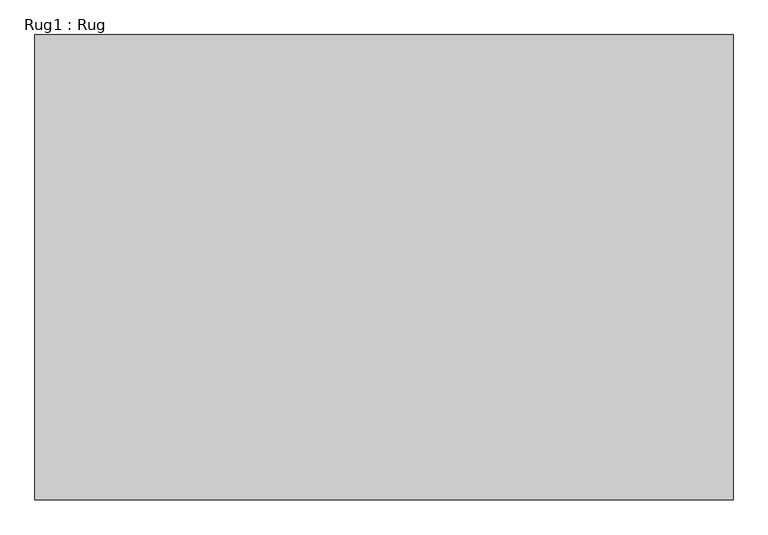
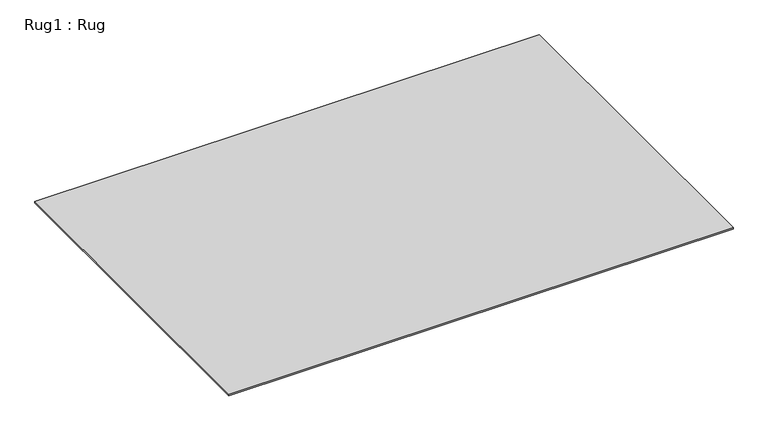
"""IFC4 building model written with IfcOpenShell, lengths in millimetres: furniture geometry, Rug1 : Rug."""

from ifc_helpers import new_model, si_unit, origin, origin_with_axes, place, context, project, spatial, polyline, outline, extrude, source, transform, mapped, element, save


def rug1_rug_774cf3d5(model_context):
    return source(origin(), model_context, "Body", "SweptSolid", [
        extrude(outline(polyline([(1500.0, 1000.0), (1500.0, -1000.0), (-1500.0, -1000.0), (-1500.0, 1000.0), (1500.0, 1000.0)])), origin_with_axes(), (0.0, 0.0, 1.0), 10.0),
    ])


if __name__ == "__main__":
    model = new_model("IFC4")
    model_context = context("Model", 3, world=origin())
    ifc_project = project(units=[si_unit("LENGTHUNIT", "METRE", prefix="MILLI")], contexts=[model_context])
    site = spatial("IfcSite", under=ifc_project)
    building = spatial("IfcBuilding", under=site)
    placement = place(None, origin())
    rug1_rug_shape = rug1_rug_774cf3d5(model_context)
    element("IfcFurniture", 1, ObjectType="Rug1 : Rug", at=placement, inside=building, context=model_context, shape_type="MappedRepresentation", body=[
        mapped(rug1_rug_shape, transform((0.0, 0.0, 0.0), x_axis=(1.0, 0.0, 0.0), y_axis=(0.0, 1.0, 0.0), z_axis=(0.0, 0.0, 1.0))),
    ])
    save(model, "model.ifc")

# Revit data of these elements
# Type "Rug1 : Rug"
#   boarder [instance default] = 100 mm
#   W [instance default] = 3000 mm
#   D [instance default] = 2000 mm
#   Boarder_2 [instance default] = no
#   main material [instance default] = Rug main
#   boarder material [instance default] = Rug Boarder
#   Default Elevation = 0
# Element 1 (IfcFurniture, "Rug1 : Rug")
#   Materials on its faces: "Rug main"
# Materials
#   "Rug main": class "Generic", colour RGB 120 120 120, transparency 0, Cost = 0
#   "Rug Boarder": class "Generic", colour RGB 120 120 120, transparency 0, Cost = 0
